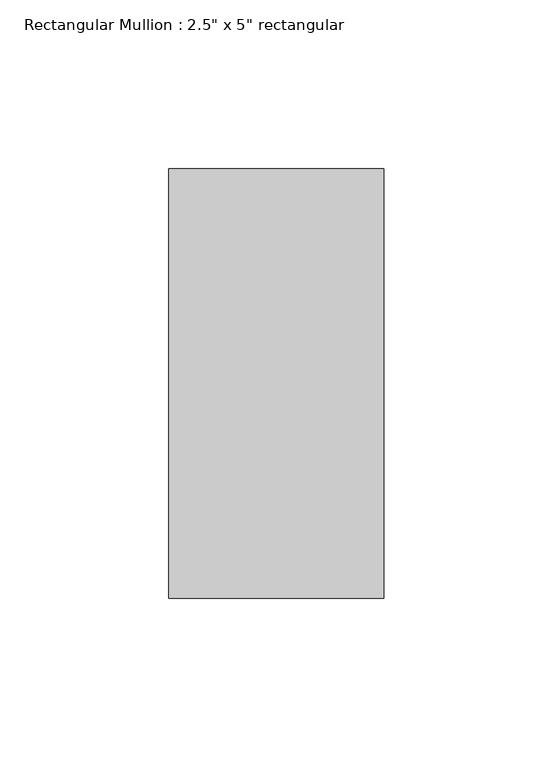
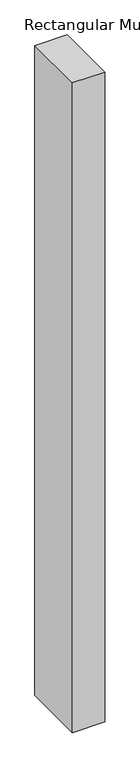
"""IFC4 building model written with IfcOpenShell, lengths in millimetres: member geometry."""

from ifc_helpers import new_model, si_unit, frame, origin, place, context, project, spatial, polyline, outline, extrude, source, transform, mapped, element, save


def member_0c868e12(model_context):
    return source(origin(), model_context, "Body", "SweptSolid", [
        extrude(outline(polyline([(0.0, 63.5), (0.0, -63.5), (-63.5, -63.5), (-63.5, 63.5), (0.0, 63.5)])), frame((0.0, 0.0, -1343.8826511), z_axis=(0.0, 0.0, 1.0), x_axis=(1.0, 0.0, 0.0)), (0.0, 0.0, 1.0), 1343.8826511),
    ])


if __name__ == "__main__":
    model = new_model("IFC4")
    model_context = context("Model", 3, world=origin())
    ifc_project = project(units=[si_unit("LENGTHUNIT", "METRE", prefix="MILLI")], contexts=[model_context])
    site = spatial("IfcSite", under=ifc_project)
    building = spatial("IfcBuilding", under=site)
    placement = place(None, origin())
    member_shape = member_0c868e12(model_context)
    element("IfcMember", 1, ObjectType="Rectangular Mullion : 2.5\" x 5\" rectangular", at=placement, inside=building, context=model_context, shape_type="MappedRepresentation", body=[
        mapped(member_shape, transform((0.0, 0.0, 0.0), x_axis=(1.0, 0.0, 0.0), y_axis=(0.0, 1.0, 0.0), z_axis=(0.0, 0.0, 1.0))),
    ])
    save(model, "model.ifc")

# Revit data of these elements
# Type "Rectangular Mullion : 2.5\" x 5\" rectangular"
#   built-in parameter 1007304 = 0.416667 (stored number, unit not read)
#   built-in parameter 1007301 = 0.104167 (stored number, unit not read)
#   built-in parameter 1007300 = 0.104167 (stored number, unit not read)
# Element 1 (IfcMember, "Rectangular Mullion : 2.5\" x 5\" rectangular")
#   Materials on its faces: "Iron, Ductile"
# Materials
#   "Iron, Ductile": class "Metal", colour RGB 0 0 0, transparency 0, Description = "Ductile cast iron", Cost = 0
